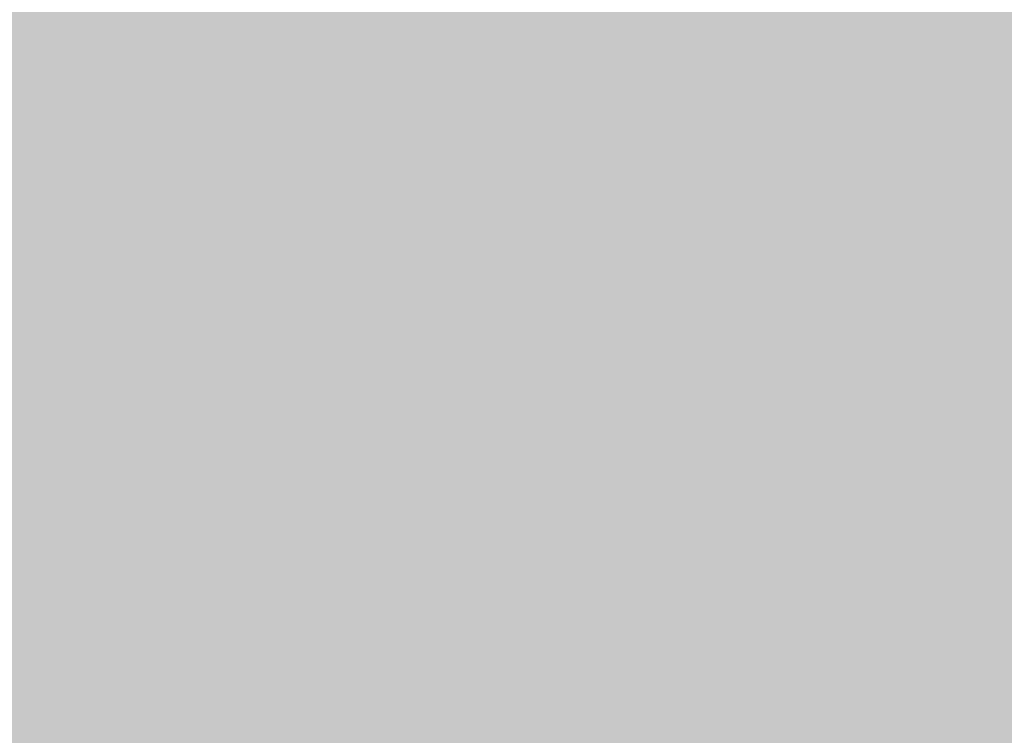
# Model space of a CAD drawing. Units: feet. Extents: x 3168 to 4724, y 827 to 1477.
# Tile 48 of 256: x 3273.072 to 3277.376, y 1093.654 to 1096.781. Entities that reach past the tile are written whole.
import ezdxf

# ---------------------------------------------------------------- set-up
doc = ezdxf.new("R2010")
doc.units = ezdxf.units.FT
doc.layers.add('A-ELEV-PATT', color=8, linetype='Continuous', lineweight=13)

msp = doc.modelspace()

# ---------------------------------------------------------------- hatches: boundary and pattern name
at = {"layer": 'A-ELEV-PATT'}
h = msp.add_hatch(color=256, dxfattribs=at)
h.dxf.hatch_style = 1
edge = h.paths.add_edge_path()
edge.add_ellipse((3552.9058, 979.2201), major_axis=(36.7449, 0), ratio=0.4848485, start_angle=0, end_angle=360)
edge = h.paths.add_edge_path()
edge.add_ellipse((3559.8916, 929.2523), major_axis=(36.7449, 0), ratio=0.4848485, start_angle=0, end_angle=360)
edge = h.paths.add_edge_path()
edge.add_line((3299.3168, 1198.6061), (3479.9167, 1198.6061))
edge.add_line((3479.9167, 1198.6061), (3479.9167, 1209.8686))
edge.add_spline(control_points=[(3479.9167, 1209.8686), (3464.3012, 1209.8686), (3448.6856, 1209.8686), (3410.9491, 1209.8686), (3388.8282, 1209.8686), (3355.6469, 1209.8686), (3344.5864, 1209.8686), (3327.9957, 1209.8686), (3322.4655, 1209.8686), (3314.1702, 1209.8686), (3311.4051, 1209.8686), (3307.2574, 1209.8686), (3305.8748, 1209.8686), (3303.801, 1209.8686), (3303.1097, 1209.8686), (3302.0728, 1209.8686), (3301.7272, 1209.8686), (3301.2087, 1209.8686), (3301.0359, 1209.8686), (3300.7767, 1209.8686), (3300.6903, 1209.8686), (3300.5606, 1209.8686), (3300.5174, 1209.8686), (3300.4526, 1209.8686), (3300.431, 1209.8686), (3300.3986, 1209.8686), (3300.3878, 1209.8686), (3300.3662, 1209.8686), (3300.3457, 1209.8686), (3300.3455, 1209.8686), (3300.3455, 1209.8686), (3300.3433, 1209.8686), (3300.3411, 1209.8686), (3300.3379, 1209.8686), (3300.3368, 1209.8686), (3300.3339, 1209.8686), (3300.3321, 1209.8686), (3300.3255, 1209.8686), (3300.3207, 1209.8686), (3300.3109, 1209.8686), (3300.306, 1209.8686), (3300.2905, 1209.8686), (3300.28, 1209.8686), (3300.2324, 1209.8688), (3300.1953, 1209.869), (3299.9511, 1209.8706), (3299.7448, 1209.8743), (3299.4368, 1209.8833), (3299.3344, 1209.8868), (3299.1811, 1209.8929), (3299.13, 1209.8951), (3298.6522, 1209.9168), (3298.2295, 1209.9457), (3297.6016, 1210.0024), (3297.3934, 1210.0235), (3297.0827, 1210.0583), (3296.9793, 1210.0705), (3296.293, 1210.1549), (3295.7181, 1210.2434), (3294.8687, 1210.3989), (3294.5877, 1210.4545), (3294.1693, 1210.5433), (3294.0304, 1210.5739), (3291.7071, 1211.1012), (3289.6536, 1211.8134), (3285.7763, 1213.564), (3283.9514, 1214.6035), (3280.5122, 1216.9801), (3278.8972, 1218.3176), (3276.3799, 1220.8295), (3275.416, 1221.9177), (3274.0393, 1223.7077), (3273.581, 1224.3495), (3273.1432, 1225.0163)], knot_values=[39.119033, 39.119033, 39.119033, 39.119033, 39.286353, 39.286353, 39.523379, 39.523379, 39.641892, 39.641892, 39.701148, 39.701148, 39.730777, 39.730777, 39.745591, 39.745591, 39.752998, 39.752998, 39.756701, 39.756701, 39.758553, 39.758553, 39.759479, 39.759479, 39.759942, 39.759942, 39.760173, 39.760173, 39.760289, 39.760289, 39.760405, 39.760405, 39.760463, 39.760463, 39.763389, 39.763389, 39.764851, 39.764851, 39.767304, 39.767304, 39.773825, 39.773825, 39.78057, 39.78057, 39.79477, 39.79477, 39.845194, 39.845194, 40.126715, 40.126715, 40.267476, 40.267476, 40.337856, 40.337856, 40.927023, 40.927023, 41.221606, 41.221606, 41.368898, 41.368898, 42.202622, 42.202622, 42.619485, 42.619485, 42.827916, 42.827916, 46.118323, 46.118323, 49.408731, 49.408731, 52.699139, 52.699139, 54.927489, 54.927489, 56.104228, 56.104228, 56.104228, 56.104228], weights=[1, 1, 1, 1, 1, 1, 1, 1, 1, 1, 1, 1, 1, 1, 1, 1, 1, 1, 1, 1, 1, 1, 1, 1, 1, 1, 1, 1, 1, 1, 1, 1, 1, 1, 1, 1, 1, 1, 1, 1, 1, 1, 1, 1, 1, 1, 1, 1, 1, 1, 1, 1, 1, 1, 1, 1, 1, 1, 1, 1, 1, 1, 1, 1, 1, 1, 1, 1, 1, 1, 1, 1, 1, 1], degree=3, periodic=0)
edge.add_line((3273.1432, 1225.0163), (3273.1432, 1099.0163))
edge.add_line((3273.1432, 1099.0163), (3299.3168, 1099.0163))
edge.add_line((3299.3168, 1099.0163), (3299.3168, 1198.6061))
edge = h.paths.add_edge_path()
edge.add_line((3304.7584, 1324.1581), (3479.9167, 1324.1581))
edge.add_line((3479.9167, 1324.1581), (3479.9167, 1335.7146))
edge.add_line((3479.9167, 1335.7146), (3269.1616, 1335.7146))
edge.add_spline(control_points=[(3269.1616, 1335.7146), (3264.0242, 1335.7146), (3258.3641, 1328.9582), (3259.2643, 1323.9003)], knot_values=[0, 0, 0, 0, 15.412191, 15.412191, 15.412191, 15.412191], degree=3, periodic=0)
edge.add_line((3259.2643, 1323.9003), (3265.5168, 1288.7691))
edge.add_line((3265.5168, 1288.7691), (3275.2651, 1261.5456))
edge.add_line((3275.2651, 1261.5456), (3304.7584, 1261.5456))
edge.add_line((3304.7584, 1261.5456), (3304.7584, 1324.1581))
h = msp.add_hatch(color=256, dxfattribs=at)
h.dxf.hatch_style = 1
h.paths.add_polyline_path([(3384.5252, 1099.0163), (3335.0292, 1099.0163), (3299.3168, 1099.0163), (3273.1432, 1099.0163), (3217.5654, 1099.0163), (3168.0693, 827.1163), (3335.0292, 827.1163)])

doc.saveas('drawing.dxf')
